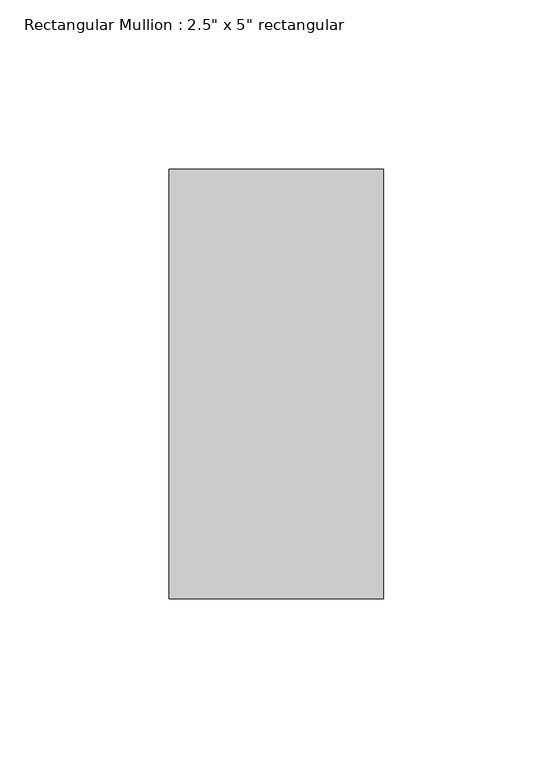
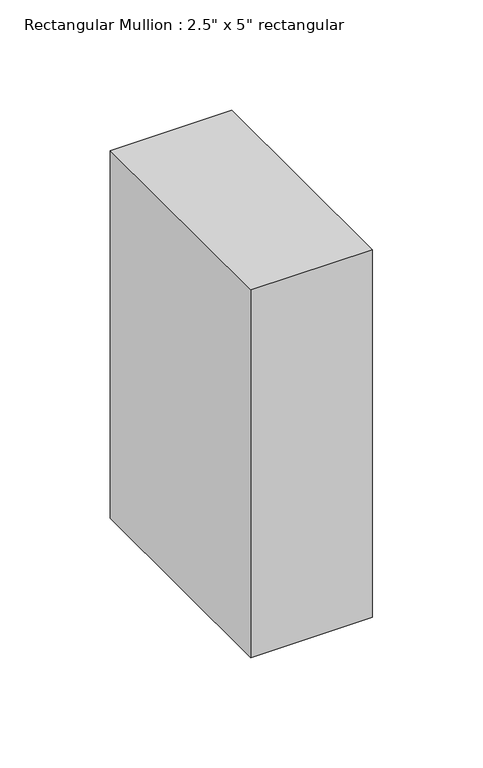
"""IFC4 building model written with IfcOpenShell, lengths in millimetres: member geometry."""

from ifc_helpers import new_model, si_unit, frame, origin, place, context, project, spatial, polyline, outline, extrude, source, transform, mapped, element, save


def member_3572ee78(model_context):
    return source(origin(), model_context, "Body", "SweptSolid", [
        extrude(outline(polyline([(31.75, 63.5), (31.75, -63.5), (-31.75, -63.5), (-31.75, 63.5), (31.75, 63.5)])), frame((0.0, 0.0, -203.2), z_axis=(0.0, 0.0, 1.0), x_axis=(1.0, 0.0, 0.0)), (0.0, 0.0, 1.0), 203.2),
    ])


if __name__ == "__main__":
    model = new_model("IFC4")
    model_context = context("Model", 3, world=origin())
    ifc_project = project(units=[si_unit("LENGTHUNIT", "METRE", prefix="MILLI")], contexts=[model_context])
    site = spatial("IfcSite", under=ifc_project)
    building = spatial("IfcBuilding", under=site)
    placement = place(None, origin())
    member_shape = member_3572ee78(model_context)
    element("IfcMember", 1, ObjectType="Rectangular Mullion : 2.5\" x 5\" rectangular", at=placement, inside=building, context=model_context, shape_type="MappedRepresentation", body=[
        mapped(member_shape, transform((0.0, 0.0, 0.0), x_axis=(1.0, 0.0, 0.0), y_axis=(0.0, 1.0, 0.0), z_axis=(0.0, 0.0, 1.0))),
    ])
    save(model, "model.ifc")

# Revit data of these elements
# Type "Rectangular Mullion : 2.5\" x 5\" rectangular"
#   built-in parameter 1007304 = 0.416667 (stored number, unit not read)
#   built-in parameter 1007301 = 0.104167 (stored number, unit not read)
#   built-in parameter 1007300 = 0.104167 (stored number, unit not read)
# Element 1 (IfcMember, "Rectangular Mullion : 2.5\" x 5\" rectangular")
#   Materials on its faces: "Aluminum"
# Materials
#   "Aluminum": class "Metal", colour RGB 247 247 247, transparency 0, Description = "Aluminum 6061", Cost = 0
